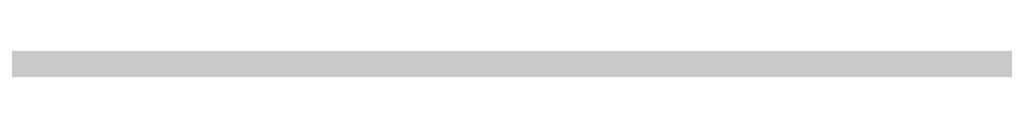
# Model space of a CAD drawing. Units: inches. Extents: x 2091 to 2899, y 967 to 2217.
# Tile 214 of 256: x 2203.2571 to 2203.4104, y 1152.2487 to 1152.2504. Entities that reach past the tile are written whole.
import ezdxf

# ---------------------------------------------------------------- set-up
doc = ezdxf.new("R2010")
doc.units = ezdxf.units.IN
doc.layers.add('A-WALL-PATT', color=141, linetype='Continuous', lineweight=13, true_color=0xadddf7)

msp = doc.modelspace()

# ---------------------------------------------------------------- hatches: boundary and pattern name
at = {"layer": 'A-WALL-PATT'}
h = msp.add_hatch(color=256, dxfattribs=at)
h.dxf.hatch_style = 1
h.paths.add_polyline_path([(2803.1436, 2050.91906), (2203.1436, 2050.91906), (2203.1436, 1090.91906), (2803.1436, 1090.91906)])
h.paths.add_polyline_path([(2635.79885, 1147.54046), (2674.52405, 1147.54046, 0.376086), (2678.52967, 1152.8802), (2678.52967, 1159.55647, 0.333335), (2674.52432, 1163.56185), (2674.52432, 1163.56185), (2674.52432, 1192.93439), (2635.80597, 1192.93439), (2597.08762, 1192.93439), (2597.08762, 1163.56185, 0.333335), (2593.08228, 1159.55647), (2593.08228, 1152.8802, 0.376086), (2597.08789, 1147.54046)], flags=0)
h.paths.add_polyline_path([(2436.01043, 1278.24078, 0.000483), (2435.95264, 1278.21503, -0.001328), (2435.93563, 1278.11169, -0.001711), (2436.11644, 1278.04076, 0.002185)], flags=0)
h.paths.add_polyline_path([(2794.1436, 1143.41906), (2794.1436, 1347.41906), (2543.37017, 1347.41906), (2543.37017, 1351.91906), (2794.1436, 1351.91906), (2794.1436, 1392.71355), (2793.9474, 1392.71355), (2793.9474, 1473.5369), (2794.1436, 1473.5369), (2794.1436, 1531.91906), (2650.1436, 1531.91906), (2650.1436, 1536.41906), (2794.1436, 1536.41906), (2794.1436, 1692.41906), (2609.37561, 1692.41906), (2609.37561, 1644.41906), (2604.87561, 1644.41906), (2604.87561, 1744.91906), (2609.37561, 1744.91906), (2609.37561, 1696.91906), (2794.1436, 1696.91906), (2794.1436, 1780.91906), (2609.6436, 1780.91906), (2493.87561, 1780.91906), (2493.87561, 1785.41906), (2609.6436, 1785.41906), (2794.1436, 1785.41906), (2794.1436, 1847.93882), (2793.95122, 1847.93882), (2793.95122, 1928.76217), (2794.1436, 1928.76217), (2794.1436, 1941.41906), (2614.1436, 1941.41906), (2614.1436, 1821.41906), (2609.6436, 1821.41906), (2609.6436, 1941.41906), (2392.1436, 1941.41906), (2392.1436, 1819.91906), (2387.6436, 1819.91906), (2387.6436, 1941.41906), (2212.1436, 1941.41906), (2212.1436, 1783.91906), (2392.1436, 1783.91906), (2392.1436, 1780.91906), (2212.1436, 1780.91906), (2212.1436, 1629.41906), (2387.6436, 1629.41906), (2387.6436, 1744.91906), (2392.1436, 1744.91906), (2392.1436, 1627.91906), (2317.1436, 1627.91906), (2317.1436, 1551.41906), (2317.1436, 1536.41906), (2459.38359, 1536.41906), (2459.38359, 1602.39648), (2463.88359, 1602.39648), (2463.88359, 1531.91906), (2456.6436, 1531.91906), (2456.6436, 1529.91906), (2452.1436, 1529.91906), (2452.1436, 1531.91906), (2312.6436, 1531.91906), (2312.6436, 1551.41906), (2306.1436, 1551.41906), (2306.1436, 1555.91906), (2308.1436, 1555.91906), (2308.1436, 1551.41906), (2312.6436, 1551.41906), (2312.6436, 1627.91906), (2212.1436, 1627.91906), (2212.1436, 1555.91906), (2270.1436, 1555.91906), (2270.1436, 1551.41906), (2212.1436, 1551.41906), (2212.1436, 1351.91906), (2272.1436, 1351.91906), (2272.1436, 1347.41906), (2212.1436, 1347.41906), (2212.1436, 1275.41906), (2308.1436, 1275.41906), (2308.1436, 1351.91906), (2452.1436, 1351.91906), (2452.1436, 1493.91906), (2456.6436, 1493.91906), (2456.6436, 1347.41906), (2312.6436, 1347.41906), (2312.6436, 1270.91906), (2212.1436, 1270.91906), (2212.1436, 1099.91906), (2281.23752, 1099.91906), (2282.87104, 1110.9138), (2282.00834, 1116.9966), (2278.55774, 1121.4204), (2268.20564, 1128.0562), (2272.08764, 1128.0562), (2273.81294, 1131.927), (2279.42034, 1134.6919), (2285.02784, 1135.2449), (2287.61584, 1137.4568), (2288.04714, 1138.0098), (2289.34114, 1140.7747), (2291.06654, 1139.6687), (2292.36054, 1135.2449), (2295.37984, 1136.9038), (2296.24254, 1135.7979), (2297.10524, 1133.033), (2300.12464, 1138.0098), (2303.14394, 1138.0098), (2304.43794, 1135.7979), (2303.14394, 1133.586), (2306.59464, 1134.6919), (2307.88874, 1133.033), (2310.90804, 1135.2449), (2313.92744, 1134.1389), (2315.62686, 1132.4271), (2308.32004, 1117.5496), (2290.20384, 1109.8079), (2288.90984, 1103.1721), (2289.27231, 1099.91906), (2434.91823, 1099.91906), (2431.59323, 1124.78806), (2429.93023, 1169.55306), (2430.92718, 1240.51969), (2435.65893, 1238.18613), (2437.13523, 1196.55406), (2438.79823, 1143.97306), (2442.67823, 1111.99806), (2446.55823, 1099.91906), (2794.1436, 1099.91906), (2794.1436, 1138.91906), (2548.03245, 1138.91906), (2548.03245, 1143.41906), (2548.03245, 1148.81906), (2546.66846, 1148.03156), (2528.68569, 1179.17862, 0.256256), (2512.03245, 1148.81906), (2512.03245, 1143.41906), (2512.03245, 1138.91906), (2507.53245, 1138.91906), (2507.53245, 1143.41906), (2507.53245, 1148.81906, 0.256256), (2490.8792, 1179.17862), (2472.89644, 1148.03156), (2471.53245, 1148.81906), (2471.53245, 1143.41906), (2467.03245, 1143.41906), (2467.03245, 1269.94579, 0.039061), (2460.90999, 1273.58006), (2467.03245, 1273.58006), (2467.03245, 1286.32536, 0.014511), (2465.21619, 1286.76191), (2467.03245, 1287.05258), (2467.03245, 1323.41906), (2471.53245, 1323.41906), (2471.53245, 1148.81906), (2489.53245, 1179.99597), (2490.89644, 1179.20847), (2490.8792, 1179.17862, -0.256256), (2507.53245, 1148.81906), (2507.53245, 1143.41906), (2512.03245, 1143.41906), (2512.03245, 1148.81906, -0.256256), (2528.68569, 1179.17862), (2528.66846, 1179.20847), (2530.03245, 1179.99597), (2548.03245, 1148.81906), (2548.03245, 1143.41906)], flags=16)
h.paths.add_polyline_path([(2607.76855, 1200.94508), (2607.76855, 1265.03063), (2597.08762, 1281.05201), (2619.78459, 1281.05201), (2627.79528, 1337.12686), (2635.79885, 1337.12686), (2643.81666, 1337.12686), (2651.82736, 1281.05201), (2674.52432, 1281.05201), (2663.8434, 1265.03063), (2663.8434, 1200.94508), (2635.80597, 1200.94508)], flags=0)
edge = h.paths.add_edge_path(flags=0)
edge.add_ellipse((13303.89622, 1272.99872), major_axis=(-10595.31304, 0), ratio=0.84230387009, start_angle=0.628237219, end_angle=0.6465541, ccw=False)
edge.add_ellipse((2711.70045, 1156.85268), major_axis=(2.21977, 0), ratio=0.8423039, start_angle=111.53524, end_angle=180.62824, ccw=False)
edge.add_ellipse((13303.15629, 1272.99872), major_axis=(-10593.02631, 0), ratio=0.84230386954, start_angle=0.528271472, end_angle=0.646554097, ccw=False)
edge.add_line((2710.7646, 1175.3333), (2710.12999, 1175.3333))
edge.add_ellipse((2710.12999, 1176.57978), major_axis=(1.47985, 0), ratio=0.8423039, start_angle=180, end_angle=270, ccw=False)
edge.add_line((2708.65014, 1176.57978), (2708.65014, 1200.78291))
edge.add_ellipse((2710.12999, 1200.78291), major_axis=(1.47985, 0), ratio=0.8423039, start_angle=90, end_angle=180, ccw=False)
edge.add_line((2710.12999, 1202.02939), (2710.46508, 1202.02939))
edge.add_ellipse((13303.15629, 1272.99872), major_axis=(-10593.02631, 0), ratio=0.84230386954, start_angle=-0.090229089, end_angle=0.383866779, ccw=False)
edge.add_ellipse((2710.12999, 1290.92703), major_axis=(-1.47985, 0), ratio=0.8423039, start_angle=0, end_angle=90, ccw=False)
edge.add_line((2708.65014, 1290.92703), (2708.65014, 1315.13017))
edge.add_ellipse((2710.12999, 1315.13017), major_axis=(-1.47985, 0), ratio=0.8423039, start_angle=-90, end_angle=0, ccw=False)
edge.add_line((2710.12999, 1316.37665), (2710.70631, 1316.37665))
edge.add_ellipse((3238.40172, 1296.28957), major_axis=(528.234, 0), ratio=0.84230387, start_angle=176.3495724, end_angle=177.8200497, ccw=False)
edge.add_ellipse((2775.06304, 1071.4507), major_axis=(313.30776, 0), ratio=0.84230387, start_angle=102.1259656, end_angle=103.780529, ccw=False)
edge.add_ellipse((2775.06304, 1078.3057), major_axis=(-305.30289, 0), ratio=0.84230387, start_angle=-79.790461, end_angle=-77.5553727, ccw=False)
edge.add_ellipse((2695.14177, 1541.97538), major_axis=(-250.96022, 0), ratio=0.84230387, start_angle=99.256566, end_angle=102.5549326)
edge.add_line((2741.41033, 1334.21426), (2747.13255, 1337.37848))
edge.add_ellipse((2747.53862, 1336.85748), major_axis=(-0.73992, 0), ratio=0.842304, start_angle=270, end_angle=307.93313, ccw=False)
edge.add_ellipse((2747.53862, 1336.85748), major_axis=(-0.73992, 0), ratio=0.842304, start_angle=232.06687, end_angle=270, ccw=False)
edge.add_line((2747.94469, 1337.37848), (2753.66691, 1334.21426))
edge.add_ellipse((2799.93547, 1541.97538), major_axis=(250.96022, 0), ratio=0.84230387, start_angle=257.4450674, end_angle=260.743434)
edge.add_ellipse((2720.01419, 1078.3057), major_axis=(305.30289, 0), ratio=0.84230387, start_angle=77.5553727, end_angle=79.790461, ccw=False)
edge.add_ellipse((2720.01419, 1071.4507), major_axis=(-313.30776, 0), ratio=0.84230387, start_angle=256.219471, end_angle=257.8740344, ccw=False)
edge.add_ellipse((2256.67551, 1296.28957), major_axis=(-528.234, 0), ratio=0.84230387, start_angle=182.1799503, end_angle=183.6504276, ccw=False)
edge.add_line((2784.37092, 1316.37665), (2784.94725, 1316.37665))
edge.add_ellipse((2784.94725, 1315.13017), major_axis=(1.47985, 0), ratio=0.8423039, start_angle=0, end_angle=90, ccw=False)
edge.add_line((2786.42709, 1315.13017), (2786.42709, 1290.92703))
edge.add_ellipse((2784.94725, 1290.92703), major_axis=(1.47985, 0), ratio=0.8423039, start_angle=270, end_angle=360, ccw=False)
edge.add_ellipse((-7808.07906, 1272.99872), major_axis=(10593.02631, 0), ratio=0.84230386954, start_angle=-0.383866779, end_angle=0.090229089, ccw=False)
edge.add_line((2784.61216, 1202.02939), (2784.94725, 1202.02939))
edge.add_ellipse((2784.94725, 1200.78291), major_axis=(1.47985, 0), ratio=0.8423039, start_angle=0, end_angle=90, ccw=False)
edge.add_line((2786.42709, 1200.78291), (2786.42709, 1176.57978))
edge.add_ellipse((2784.94725, 1176.57978), major_axis=(-1.47985, 0), ratio=0.8423039, start_angle=90, end_angle=180, ccw=False)
edge.add_line((2784.94725, 1175.3333), (2784.31264, 1175.3333))
edge.add_ellipse((-7808.07906, 1272.99872), major_axis=(10593.02631, 0), ratio=0.84230386954, start_angle=-0.618643196, end_angle=-0.528271472, ccw=False)
edge.add_ellipse((2783.37678, 1156.85268), major_axis=(-2.21977, 0), ratio=0.8423039, start_angle=179.37176, end_angle=248.46476, ccw=False)
edge.add_ellipse((-7808.81898, 1272.99872), major_axis=(-10595.31304, 0), ratio=0.84230386576, start_angle=179.353445923, end_angle=179.371762803, ccw=False)
edge.add_ellipse((2780.2973, 1153.50079), major_axis=(-5.24643, 0), ratio=0.8423039, start_angle=90, end_angle=179.35345, ccw=False)
edge.add_line((2780.2973, 1149.08171), (2714.77993, 1149.08171))
edge.add_ellipse((2714.77993, 1153.50079), major_axis=(5.24643, 0), ratio=0.8423039, start_angle=180.64655, end_angle=270, ccw=False)
edge = h.paths.add_edge_path(flags=0)
edge.add_line((2718.18737, 1151.00783), (2718.18737, 1170.47236))
edge.add_ellipse((2721.14706, 1170.47236), major_axis=(-2.95969, 0), ratio=0.8423039, start_angle=-90, end_angle=0, ccw=False)
edge.add_line((2721.14706, 1172.96532), (2773.93017, 1172.96532))
edge.add_ellipse((2773.93017, 1170.47236), major_axis=(-2.95969, 0), ratio=0.8423039, start_angle=180, end_angle=270, ccw=False)
edge.add_line((2776.88987, 1170.47236), (2776.88987, 1151.00783))
edge.add_line((2776.88987, 1151.00783), (2718.18737, 1151.00783))
edge = h.paths.add_edge_path(flags=0)
edge.add_line((2718.18737, 1180.23415), (2718.18737, 1199.05783))
edge.add_ellipse((2747.53862, 1320.39864), major_axis=(147.01792, 0), ratio=0.84230387, start_angle=256.4018653, end_angle=283.5981347)
edge.add_line((2776.88987, 1199.05783), (2776.88987, 1180.23415))
edge.add_ellipse((2747.53862, 1301.57496), major_axis=(147.01792, 0), ratio=0.84230387, start_angle=256.4018653, end_angle=283.5981347, ccw=False)
edge = h.paths.add_edge_path(flags=0)
edge.add_ellipse((13303.15629, 1272.99872), major_axis=(-10591.54646, 0), ratio=0.84230386955, start_angle=0.055594314, end_angle=0.377764194, ccw=False)
edge.add_line((2711.61686, 1262.72171), (2715.66741, 1249.4954))
edge.add_ellipse((6413.89196, 1241.69192), major_axis=(-3698.23616, 0), ratio=0.8423038695, start_angle=-0.12089737, end_angle=0.36407635)
edge.add_line((2715.76104, 1218.19245), (2711.93431, 1203.16736))
edge = h.paths.add_edge_path(flags=0)
edge.add_line((2718.18737, 1251.07457), (2716.00249, 1267.45044))
edge.add_ellipse((2742.15117, 1202.18954), major_axis=(81.77258, 0), ratio=0.84230387, start_angle=94.277421, end_angle=111.8349538, ccw=False)
edge.add_line((2737.00975, 1270.93063), (2758.06748, 1270.93063))
edge.add_ellipse((2752.92606, 1202.18954), major_axis=(81.77258, 0), ratio=0.84230387, start_angle=68.1650462, end_angle=85.722579, ccw=False)
edge.add_line((2779.07475, 1267.45044), (2776.88987, 1251.07457))
edge.add_ellipse((2750.33806, 1187.88536), major_axis=(79.57966, 0), ratio=0.84230387, start_angle=67.2080851, end_angle=85.1299304)
edge.add_line((2756.03466, 1254.74366), (2739.04258, 1254.74366))
edge.add_ellipse((2744.73917, 1187.88536), major_axis=(79.57966, 0), ratio=0.84230387, start_angle=94.8700696, end_angle=112.7919149)
edge = h.paths.add_edge_path(flags=0)
edge.add_line((2783.14293, 1203.16736), (2779.31619, 1218.19245))
edge.add_ellipse((-918.81473, 1241.69192), major_axis=(3698.23616, 0), ratio=0.8423038695, start_angle=-0.36407635, end_angle=0.12089737)
edge.add_line((2779.40983, 1249.4954), (2783.46037, 1262.72171))
edge.add_ellipse((-7808.07906, 1272.99872), major_axis=(-10591.54646, 0), ratio=0.84230386954, start_angle=179.622235806, end_angle=179.944405687, ccw=False)
edge = h.paths.add_edge_path(flags=0)
edge.add_ellipse((2734.20089, 1286.69044), major_axis=(-0.35661, 6.34008), ratio=0.6038336, start_angle=89.002014, end_angle=253.657408, ccw=False)
edge.add_line((2730.369, 1286.54181), (2730.369, 1301.35198))
edge.add_line((2730.369, 1301.35198), (2735.91331, 1305.2148))
edge.add_ellipse((2736.38492, 1304.73456), major_axis=(0.73992, 0), ratio=0.842304, start_angle=90, end_angle=134.48021, ccw=False)
edge.add_line((2736.38492, 1305.3578), (2738.03278, 1305.3578))
edge.add_line((2738.03278, 1305.3578), (2738.03278, 1307.70793))
edge.add_ellipse((2794.20164, 1307.70793), major_axis=(56.16886, 0), ratio=0.84230387, start_angle=150.56143, end_angle=180, ccw=False)
edge.add_ellipse((2700.87559, 1307.70793), major_axis=(-56.16886, 0), ratio=0.84230387, start_angle=180, end_angle=209.43857, ccw=False)
edge.add_line((2757.04445, 1307.70793), (2757.04445, 1305.3578))
edge.add_line((2757.04445, 1305.3578), (2758.69232, 1305.3578))
edge.add_ellipse((2758.69232, 1304.73456), major_axis=(-0.73992, 0), ratio=0.842304, start_angle=225.51979, end_angle=270, ccw=False)
edge.add_line((2759.16392, 1305.2148), (2764.70823, 1301.35198))
edge.add_line((2764.70823, 1301.35198), (2764.70823, 1286.54181))
edge.add_ellipse((2760.87634, 1286.69044), major_axis=(0.35661, 6.34008), ratio=0.6038336, start_angle=106.342592, end_angle=270.997986, ccw=False)
edge.add_line((2757.04445, 1285.79709), (2757.04445, 1307.70793))
edge.add_ellipse((2700.87559, 1307.70793), major_axis=(-56.16886, 0), ratio=0.84230387, start_angle=180, end_angle=209.43857)
edge.add_ellipse((2794.20164, 1307.70793), major_axis=(56.16886, 0), ratio=0.84230387, start_angle=150.56143, end_angle=180)
edge.add_line((2738.03278, 1307.70793), (2738.03278, 1285.79709))
h.paths.add_polyline_path([(2417.81227, 1104.4497), (2413.49227, 1102.5297), (2410.61227, 1103.9697), (2409.17227, 1106.3697), (2407.25227, 1107.3297), (2406.29227, 1109.7297), (2405.33227, 1114.0497), (2405.33227, 1117.8897), (2406.29227, 1120.1297), (2407.25227, 1119.8097), (2408.84832, 1118.32766), (2410.17395, 1119.42417), (2410.21127, 1120.4057), (2411.04073, 1121.41905), (2410.69927, 1119.8587), (2410.17395, 1119.42417), (2410.08845, 1117.17611), (2411.13284, 1116.20632), (2413.97227, 1119.3297), (2416.85227, 1120.7697), (2416.86972, 1120.79878), (2417.03507, 1119.40512), (2417.89621, 1118.14338), (2418.29227, 1118.3697), (2419.54445, 1120.03927), (2419.36092, 1118.38749), (2419.03211, 1119.35615), (2418.39894, 1118.51193), (2419.25227, 1114.5297), (2418.79409, 1107.19879)], flags=0)
h.paths.add_polyline_path([(2508.87017, 1347.41906), (2508.37017, 1347.41906), (2508.37017, 1351.91906), (2508.87017, 1351.91906)], flags=0)
h.paths.add_polyline_path([(2473.37017, 1347.41906), (2472.37017, 1347.41906), (2467.87017, 1347.41906), (2467.87017, 1455.41906), (2472.37017, 1455.41906), (2472.37017, 1352.41906), (2473.37017, 1352.41906)], flags=0)
h.paths.add_polyline_path([(2352.10624, 1217.4462), (2349.22624, 1218.8862), (2347.78624, 1221.2862), (2345.86624, 1222.2462), (2344.90624, 1224.6462), (2343.94624, 1228.9662), (2343.94624, 1232.8062), (2344.90624, 1235.0462), (2345.86624, 1234.7262), (2347.46229, 1233.24415), (2348.78792, 1234.34066), (2348.82524, 1235.3222), (2349.6547, 1236.33555), (2349.31324, 1234.7752), (2348.78792, 1234.34066), (2348.70242, 1232.0926), (2349.74681, 1231.12282), (2352.58624, 1234.2462), (2355.46624, 1235.6862), (2355.48369, 1235.71528), (2355.64904, 1234.32161), (2356.51018, 1233.05988), (2356.90624, 1233.2862), (2358.15842, 1234.95576), (2357.97489, 1233.30398), (2357.64608, 1234.27264), (2357.01291, 1233.42842), (2357.86624, 1229.4462), (2357.40806, 1222.11529), (2356.42624, 1219.3662)], flags=0)
h.paths.add_polyline_path([(2348.2968, 1112.22442), (2347.0138, 1112.31042), (2345.5298, 1114.12742), (2345.7318, 1115.85842), (2346.8118, 1116.98242), (2346.8118, 1114.64642), (2345.8668, 1114.21442), (2346.8798, 1114.30042)], flags=0)
h.paths.add_polyline_path([(2347.0138, 1110.92642), (2346.2718, 1110.49342), (2346.6098, 1111.18642)], flags=0)
h.paths.add_polyline_path([(2345.8668, 1118.19442), (2345.5298, 1117.32942), (2343.7078, 1118.02142), (2344.3828, 1118.62642)], flags=0)
h.paths.add_polyline_path([(2346.6768, 1109.28242), (2346.0698, 1108.07142), (2345.8668, 1110.06142)], flags=0)
h.paths.add_polyline_path([(2345.0568, 1119.75142), (2343.6398, 1119.75142), (2343.9778, 1121.13542)], flags=0)
h.paths.add_polyline_path([(2345.2598, 1116.55042), (2345.1248, 1115.85842), (2344.9218, 1115.68542), (2344.7198, 1116.37742)], flags=0)
h.paths.add_polyline_path([(2345.6648, 1112.31042), (2345.4618, 1111.53242), (2344.0448, 1111.96442), (2344.6518, 1112.57042)], flags=0)
h.paths.add_polyline_path([(2345.1918, 1113.34942), (2344.4498, 1113.86842), (2344.7198, 1114.38742)], flags=0)
h.paths.add_polyline_path([(2344.6518, 1116.80942), (2344.1798, 1115.68542), (2344.6518, 1115.33942), (2343.9098, 1114.90642), (2343.0328, 1115.94442), (2343.6398, 1116.46342)], flags=0)
h.paths.add_polyline_path([(2345.8668, 1106.68642), (2344.9898, 1105.56242), (2344.5168, 1106.60042)], flags=0)
h.paths.add_polyline_path([(2344.8548, 1110.06142), (2344.5168, 1109.28242), (2344.1128, 1109.71542)], flags=0)
h.paths.add_polyline_path([(2344.0448, 1113.52242), (2343.4378, 1113.08942), (2342.7628, 1113.95442)], flags=0)
h.paths.add_polyline_path([(2344.3148, 1111.01242), (2342.9648, 1110.32042), (2342.9648, 1111.09942)], flags=0)
h.paths.add_polyline_path([(2345.1248, 1104.69742), (2344.5848, 1103.74542), (2344.4498, 1104.26442)], flags=0)
h.paths.add_polyline_path([(2342.8298, 1121.22242), (2341.7498, 1120.53042), (2340.5358, 1121.04942), (2340.1308, 1121.82842), (2340.6708, 1122.95242), (2341.1428, 1121.82842), (2341.6148, 1122.00142)], flags=0)
h.paths.add_polyline_path([(2342.9648, 1119.75142), (2343.0328, 1118.45342), (2342.0878, 1118.02142), (2342.0198, 1119.49142)], flags=0)
h.paths.add_polyline_path([(2342.6948, 1116.89642), (2341.9528, 1116.63642), (2342.0198, 1117.32942)], flags=0)
h.paths.add_polyline_path([(2343.0328, 1112.22442), (2342.0198, 1111.79142), (2341.5478, 1112.22442), (2342.3578, 1113.34942)], flags=0)
h.paths.add_polyline_path([(2343.7748, 1104.43742), (2342.6278, 1102.88042), (2342.6948, 1104.61042), (2343.4378, 1105.12942)], flags=0)
h.paths.add_polyline_path([(2342.0198, 1115.07942), (2340.8058, 1115.51242), (2340.9408, 1116.37742)], flags=0)
h.paths.add_polyline_path([(2341.4808, 1120.09742), (2341.4808, 1119.40542), (2341.0758, 1119.57842), (2341.1428, 1120.09742)], flags=0)
h.paths.add_polyline_path([(2341.8178, 1114.47342), (2340.9408, 1113.08942), (2340.8058, 1114.56042)], flags=0)
h.paths.add_polyline_path([(2341.1428, 1118.54042), (2340.9408, 1116.98242), (2339.0508, 1117.67542), (2339.0508, 1118.62642)], flags=0)
h.paths.add_polyline_path([(2342.6948, 1101.66842), (2341.9528, 1101.84142), (2342.5598, 1102.36142)], flags=0)
h.paths.add_polyline_path([(2340.3328, 1119.66542), (2338.4438, 1119.57842), (2337.9038, 1120.35742), (2339.6578, 1120.61642)], flags=0)
h.paths.add_polyline_path([(2340.3328, 1115.33942), (2340.0628, 1113.69542), (2339.3878, 1115.33942)], flags=0)
h.paths.add_polyline_path([(2341.8178, 1103.83142), (2341.5478, 1102.88042), (2341.1428, 1103.65842)], flags=0)
h.paths.add_polyline_path([(2339.0508, 1122.86642), (2337.2958, 1121.82842), (2337.0938, 1123.12542), (2337.7688, 1123.81842)], flags=0)
h.paths.add_polyline_path([(2339.1178, 1121.74142), (2338.8478, 1121.22242), (2338.1738, 1121.04942), (2338.3758, 1121.56842)], flags=0)
h.paths.add_polyline_path([(2339.1858, 1119.31942), (2338.6458, 1118.71342), (2338.2408, 1118.10742), (2338.2408, 1118.88642)], flags=0)
h.paths.add_polyline_path([(2341.1428, 1101.92842), (2340.6028, 1101.23642), (2340.0628, 1101.84142), (2340.6028, 1102.36142)], flags=0)
h.paths.add_polyline_path([(2337.6338, 1117.76142), (2336.6208, 1118.28042), (2337.2958, 1118.97242)], flags=0)
h.paths.add_polyline_path([(2336.8238, 1119.57842), (2334.7988, 1118.97242), (2335.2038, 1120.35742), (2336.5538, 1120.87642)], flags=0)
h.paths.add_polyline_path([(2339.1178, 1100.45742), (2337.3638, 1100.54342), (2336.7558, 1101.23642)], flags=0)
h.paths.add_polyline_path([(2336.3508, 1122.43342), (2336.0138, 1121.91442), (2334.9338, 1122.43342), (2334.5288, 1123.47142), (2335.7438, 1122.77942)], flags=0)
h.paths.add_polyline_path([(2334.7318, 1120.87642), (2334.2588, 1120.35742), (2334.0568, 1120.78942), (2334.5968, 1121.30842)], flags=0)
h.paths.add_polyline_path([(2334.4618, 1122.17442), (2332.5718, 1121.30842), (2331.3568, 1122.17442), (2332.0998, 1122.86642)], flags=0)
h.paths.add_polyline_path([(2334.2588, 1118.54042), (2333.3818, 1118.45342), (2333.6518, 1119.31942)], flags=0)
h.paths.add_polyline_path([(2335.5418, 1102.27442), (2334.1918, 1102.62042), (2335.2718, 1103.31242)], flags=0)
h.paths.add_polyline_path([(2332.7068, 1119.66542), (2331.6948, 1120.44342), (2332.5048, 1120.78942)], flags=0)
h.paths.add_polyline_path([(2334.7318, 1101.14942), (2333.5168, 1101.58242), (2333.9888, 1101.75542)], flags=0)
h.paths.add_polyline_path([(2332.6398, 1116.63642), (2331.0868, 1116.29042), (2331.9648, 1118.19442)], flags=0)
h.paths.add_polyline_path([(2330.7498, 1121.56842), (2330.2768, 1120.27042), (2328.5228, 1119.31942), (2328.9948, 1121.04942)], flags=0)
h.paths.add_polyline_path([(2330.7498, 1118.62642), (2330.0078, 1117.50242), (2329.8728, 1118.02142)], flags=0)
h.paths.add_polyline_path([(2332.0998, 1102.36142), (2330.5468, 1102.01442), (2331.6948, 1102.96642)], flags=0)
h.paths.add_polyline_path([(2329.5348, 1113.60842), (2329.0628, 1112.31042), (2328.5898, 1113.34942)], flags=0)
h.paths.add_polyline_path([(2328.3878, 1117.84842), (2327.5098, 1116.55042), (2327.1728, 1117.76142)], flags=0)
h.paths.add_polyline_path([(2329.7378, 1106.51342), (2329.5348, 1105.30242), (2328.2528, 1106.08142)], flags=0)
h.paths.add_polyline_path([(2328.6578, 1114.38742), (2328.0498, 1114.12742), (2328.3198, 1114.90642)], flags=0)
h.paths.add_polyline_path([(2328.3198, 1112.22442), (2327.1058, 1112.13742), (2326.7008, 1112.65642)], flags=0)
h.paths.add_polyline_path([(2326.9028, 1115.25242), (2326.7008, 1114.12742), (2325.2158, 1113.60842), (2326.0928, 1115.33942)], flags=0)
h.paths.add_polyline_path([(2326.6328, 1108.33042), (2326.0928, 1107.37942), (2325.8908, 1108.50342), (2326.4978, 1109.10942)], flags=0)
h.paths.add_polyline_path([(2615.1436, 1531.91906), (2609.6436, 1531.91906), (2609.6436, 1620.41906), (2614.1436, 1620.41906), (2614.1436, 1536.41906), (2615.1436, 1536.41906)], flags=0)
h.paths.add_polyline_path([(2545.1436, 1563.41906), (2464.1436, 1563.41906), (2464.1436, 1632.41906), (2509.1436, 1632.41906), (2509.1436, 1627.91906), (2509.1436, 1603.91906), (2468.6436, 1603.91906), (2468.6436, 1567.91906), (2540.6436, 1567.91906), (2540.6436, 1591.91906), (2545.1436, 1591.91906)], flags=0)
h.paths.add_polyline_path([(2388.96905, 1549.98573), (2357.43418, 1549.98573), (2357.43418, 1623.36078), (2399.36278, 1623.36078), (2435.68947, 1623.36078), (2435.59255, 1602.55927), (2435.59255, 1602.39648), (2388.96905, 1602.39648)], flags=0)
h.paths.add_polyline_path([(2388.88063, 1555.80915), (2374.90443, 1555.80915), (2374.90443, 1600.57156), (2374.90443, 1615.45765), (2406.35088, 1615.45765), (2406.35088, 1618.93943), (2412.17429, 1615.45765), (2406.35088, 1611.97586), (2406.35088, 1615.45765), (2388.88063, 1615.45765)], flags=0)
h.paths.add_polyline_path([(2568.87561, 1644.41906), (2453.37561, 1644.41906), (2453.37561, 1785.41906), (2457.87561, 1785.41906), (2457.87561, 1648.91906), (2568.87561, 1648.91906)], flags=0)
h.paths.add_polyline_path([(2212.1436, 1945.91906), (2212.1436, 2041.91906), (2794.1436, 2041.91906), (2794.1436, 1945.91906)], flags=16)
h.paths.add_polyline_path([(2271.08273, 1964.31724), (2776.85297, 1964.31724), (2776.85297, 2037.16962), (2271.08273, 2037.16962)], flags=8)
h.paths.add_polyline_path([(2380.64929, 1536.82414), (2461.04081, 1536.82414), (2461.04081, 1554.65259), (2380.64929, 1554.65259)], flags=8)
h.paths.add_polyline_path([(2240.75571, 1609.72545), (2309.18583, 1609.72545), (2309.18583, 1617.6982), (2240.75571, 1617.6982)], flags=8)
h.paths.add_polyline_path([(2212.67726, 1313.5041), (2282.59152, 1313.5041), (2282.59152, 1322.74524), (2212.67726, 1322.74524)], flags=8)
h.paths.add_polyline_path([(2457.11198, 1114.77857), (2558.48158, 1114.77857), (2558.48158, 1142.21968), (2457.11198, 1142.21968)], flags=8)
h.paths.add_polyline_path([(2473.44234, 1273.01007), (2604.64123, 1273.01007), (2604.64123, 1318.34693), (2473.44234, 1318.34693)], flags=8)
h.paths.add_polyline_path([(2638.8763, 1626.97743), (2684.25037, 1627.97674), (2684.03848, 1637.59749), (2638.66442, 1636.59819)], flags=8)
h.paths.add_polyline_path([(2537.59055, 1453.79345), (2628.38955, 1453.79345), (2628.38955, 1475.34481), (2537.59055, 1475.34481)], flags=8)
h.paths.add_polyline_path([(2504.13764, 1714.6324), (2554.64719, 1714.6324), (2554.64719, 1730.23771), (2504.13764, 1730.23771)], flags=8)
h.paths.add_polyline_path([(2487.50118, 1575.65187), (2535.09712, 1575.65187), (2535.09712, 1598.37765), (2487.50118, 1598.37765)], flags=8)
h.paths.add_polyline_path([(2709.0994, 1735.71028), (2740.0166, 1735.71028), (2740.0166, 1749.93764), (2709.0994, 1749.93764)], flags=8)
h.paths.add_polyline_path([(2442.43842, 1792.17166), (2564.72884, 1792.17166), (2564.72884, 1842.00016), (2442.43842, 1842.00016)], flags=8)
h.paths.add_polyline_path([(2655.8158, 1809.64408), (2789.52014, 1806.6938), (2790.08498, 1832.29164), (2656.38064, 1835.24192)], flags=8)
h.paths.add_polyline_path([(2234.8427, 1797.72014), (2368.59285, 1794.76885), (2369.16072, 1820.50413), (2235.41056, 1823.45542)], flags=8)
h.paths.add_polyline_path([(2245.13847, 1644.00633), (2398.42773, 1640.6239), (2398.99484, 1666.32482), (2245.70557, 1669.70725)], flags=8)
h.paths.add_polyline_path([(2306.14285, 1431.16852), (2413.76831, 1428.79369), (2414.33315, 1454.39153), (2306.70768, 1456.76636)], flags=8)
h.paths.add_polyline_path([(2306.83458, 1458.23314), (2393.38048, 1456.32345), (2393.93281, 1481.35436), (2307.38691, 1483.26405)], flags=8)

doc.saveas('drawing.dxf')
